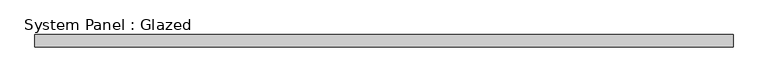
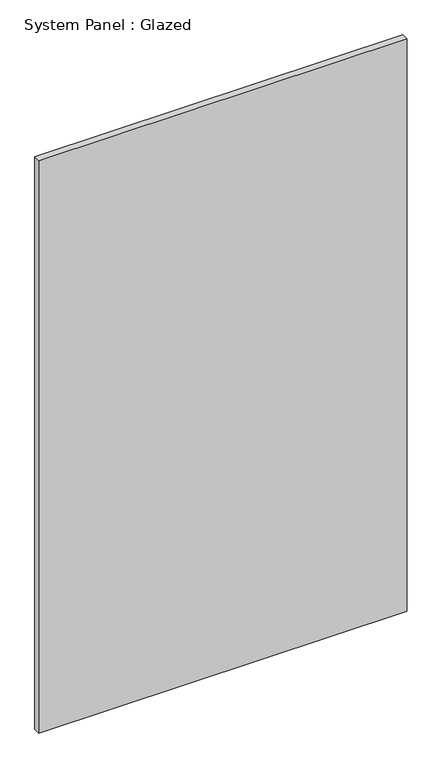
"""IFC4 building model written with IfcOpenShell, lengths in millimetres: plate geometry, System Panel : Glazed."""

from ifc_helpers import new_model, si_unit, origin, origin_with_axes, place, context, project, spatial, polyline, outline, extrude, source, transform, mapped, element, save


def system_panel_glazed_56a6bb10(model_context):
    return source(origin(), model_context, "Body", "SweptSolid", [
        extrude(outline(polyline([(713.3166667, 19.05), (-713.3166667, 19.05), (-713.3166667, 44.45), (713.3166667, 44.45), (713.3166667, 19.05)])), origin_with_axes(), (0.0, 0.0, 1.0), 2343.15),
    ])


if __name__ == "__main__":
    model = new_model("IFC4")
    model_context = context("Model", 3, world=origin())
    ifc_project = project(units=[si_unit("LENGTHUNIT", "METRE", prefix="MILLI")], contexts=[model_context])
    site = spatial("IfcSite", under=ifc_project)
    building = spatial("IfcBuilding", under=site)
    placement = place(None, origin())
    system_panel_glazed_shape = system_panel_glazed_56a6bb10(model_context)
    element("IfcPlate", 1, ObjectType="System Panel : Glazed", at=placement, inside=building, context=model_context, shape_type="MappedRepresentation", body=[
        mapped(system_panel_glazed_shape, transform((0.0, 0.0, 0.0), x_axis=(1.0, 0.0, 0.0), y_axis=(0.0, 1.0, 0.0), z_axis=(0.0, 0.0, 1.0))),
    ])
    save(model, "model.ifc")

# Revit data of these elements
# Type "System Panel : Glazed"
#   Construction Type Id = "GSP4R"
#   Analytic Construction = "1/8 in Pilkington single glazing"
#   Visual Light Transmittance = 0.9
#   Solar Heat Gain Coefficient = 0.86
#   Heat Transfer Coefficient (U) = 1.18115 BTU/(h·ft²·°F)
# Element 1 (IfcPlate, "System Panel : Glazed")
#   Materials on its faces: "Glass"
# Materials
#   "Glass": class "Glass", colour RGB 0 128 192, transparency 0.75, Description = "Soda Lime Glass", Cost = 0
